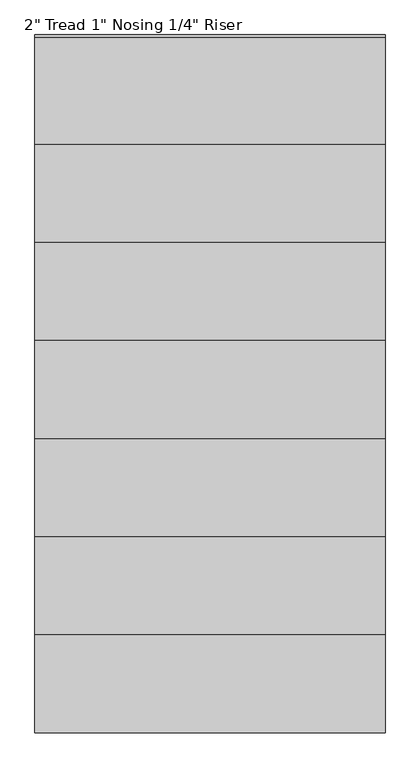
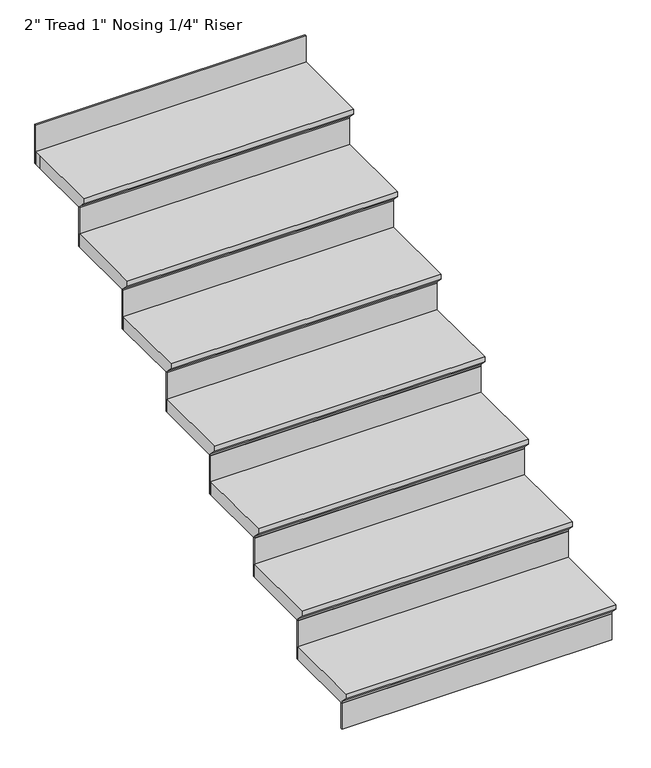
"""IFC4 building model written with IfcOpenShell, lengths in millimetres: stair flight geometry."""

from ifc_helpers import new_model, si_unit, origin, place, context, project, spatial, faceted_brep, source, transform, mapped, element, save


def stair_flight_7d9c97bb(model_context):
    return source(origin(), model_context, "Body", "Brep", [
        faceted_brep([(-6818.6502526, 9239.7128362, 3638.55), (-6818.6502526, 9239.7128362, 3657.6), (-7815.6002526, 9239.7128362, 3657.6), (-7815.6002526, 9239.7128362, 3638.55), (-6818.6502526, 9265.1128362, 3613.15), (-7815.6002526, 9265.1128362, 3613.15), (-6818.6502526, 9544.5128362, 3657.6), (-7815.6002526, 9544.5128362, 3657.6), (-7815.6002526, 9265.1128362, 3606.8), (-7815.6002526, 9544.5128362, 3606.8), (-6818.6502526, 9544.5128362, 3606.8), (-6818.6502526, 9265.1128362, 3606.8)], [[[0, 1, 2, 3]], [[4, 0, 3, 5]], [[2, 1, 6, 7]], [[8, 9, 10, 11]], [[2, 7, 9, 8, 5, 3]], [[8, 11, 4, 5]], [[6, 1, 0, 4, 11, 10]], [[7, 6, 10, 9]]]),
        faceted_brep([(-6818.6502526, 9265.1128362, 3606.8), (-6818.6502526, 9265.1128362, 3505.2), (-6818.6502526, 9271.4628362, 3505.2), (-6818.6502526, 9271.4628362, 3606.8), (-7815.6002526, 9265.1128362, 3606.8), (-7815.6002526, 9271.4628362, 3606.8), (-7815.6002526, 9271.4628362, 3505.2), (-7815.6002526, 9265.1128362, 3505.2)], [[[0, 1, 2, 3]], [[4, 5, 6, 7]], [[1, 0, 4, 7]], [[2, 1, 7, 6]], [[3, 2, 6, 5]], [[0, 3, 5, 4]]]),
        faceted_brep([(-6818.6502526, 9544.5128362, 3759.2), (-6818.6502526, 9544.5128362, 3606.8), (-6818.6502526, 9550.8628362, 3606.8), (-6818.6502526, 9550.8628362, 3759.2), (-7815.6002526, 9544.5128362, 3759.2), (-7815.6002526, 9550.8628362, 3759.2), (-7815.6002526, 9550.8628362, 3606.8), (-7815.6002526, 9544.5128362, 3606.8)], [[[0, 1, 2, 3]], [[4, 5, 6, 7]], [[1, 0, 4, 7]], [[2, 1, 7, 6]], [[3, 2, 6, 5]], [[0, 3, 5, 4]]]),
        faceted_brep([(-7815.6002526, 9519.1128362, 3810.0), (-6818.6502526, 9519.1128362, 3810.0), (-6818.6502526, 9823.9128362, 3810.0), (-7815.6002526, 9823.9128362, 3810.0), (-7815.6002526, 9544.5128362, 3759.2), (-7815.6002526, 9823.9128362, 3759.2), (-6818.6502526, 9823.9128362, 3759.2), (-6818.6502526, 9544.5128362, 3759.2), (-7815.6002526, 9544.5128362, 3765.55), (-7815.6002526, 9519.1128362, 3790.95), (-6818.6502526, 9544.5128362, 3765.55), (-6818.6502526, 9519.1128362, 3790.95)], [[[0, 1, 2, 3]], [[4, 5, 6, 7]], [[0, 3, 5, 4, 8, 9]], [[4, 7, 10, 8]], [[2, 1, 11, 10, 7, 6]], [[3, 2, 6, 5]], [[11, 1, 0, 9]], [[10, 11, 9, 8]]]),
        faceted_brep([(-6818.6502526, 9823.9128362, 3911.6), (-6818.6502526, 9823.9128362, 3759.2), (-6818.6502526, 9830.2628362, 3759.2), (-6818.6502526, 9830.2628362, 3911.6), (-7815.6002526, 9823.9128362, 3911.6), (-7815.6002526, 9830.2628362, 3911.6), (-7815.6002526, 9830.2628362, 3759.2), (-7815.6002526, 9823.9128362, 3759.2)], [[[0, 1, 2, 3]], [[4, 5, 6, 7]], [[1, 0, 4, 7]], [[2, 1, 7, 6]], [[3, 2, 6, 5]], [[0, 3, 5, 4]]]),
        faceted_brep([(-7815.6002526, 9798.5128362, 3962.4), (-6818.6502526, 9798.5128362, 3962.4), (-6818.6502526, 10103.3128362, 3962.4), (-7815.6002526, 10103.3128362, 3962.4), (-7815.6002526, 9823.9128362, 3911.6), (-7815.6002526, 10103.3128362, 3911.6), (-6818.6502526, 10103.3128362, 3911.6), (-6818.6502526, 9823.9128362, 3911.6), (-7815.6002526, 9823.9128362, 3917.95), (-7815.6002526, 9798.5128362, 3943.35), (-6818.6502526, 9823.9128362, 3917.95), (-6818.6502526, 9798.5128362, 3943.35)], [[[0, 1, 2, 3]], [[4, 5, 6, 7]], [[0, 3, 5, 4, 8, 9]], [[4, 7, 10, 8]], [[2, 1, 11, 10, 7, 6]], [[3, 2, 6, 5]], [[11, 1, 0, 9]], [[10, 11, 9, 8]]]),
        faceted_brep([(-6818.6502526, 10103.3128362, 4064.0), (-6818.6502526, 10103.3128362, 3911.6), (-6818.6502526, 10109.6628362, 3911.6), (-6818.6502526, 10109.6628362, 4064.0), (-7815.6002526, 10103.3128362, 4064.0), (-7815.6002526, 10109.6628362, 4064.0), (-7815.6002526, 10109.6628362, 3911.6), (-7815.6002526, 10103.3128362, 3911.6)], [[[0, 1, 2, 3]], [[4, 5, 6, 7]], [[1, 0, 4, 7]], [[2, 1, 7, 6]], [[3, 2, 6, 5]], [[0, 3, 5, 4]]]),
        faceted_brep([(-7815.6002526, 10077.9128362, 4114.8), (-6818.6502526, 10077.9128362, 4114.8), (-6818.6502526, 10382.7128362, 4114.8), (-7815.6002526, 10382.7128362, 4114.8), (-7815.6002526, 10103.3128362, 4064.0), (-7815.6002526, 10382.7128362, 4064.0), (-6818.6502526, 10382.7128362, 4064.0), (-6818.6502526, 10103.3128362, 4064.0), (-7815.6002526, 10103.3128362, 4070.35), (-7815.6002526, 10077.9128362, 4095.75), (-6818.6502526, 10103.3128362, 4070.35), (-6818.6502526, 10077.9128362, 4095.75)], [[[0, 1, 2, 3]], [[4, 5, 6, 7]], [[0, 3, 5, 4, 8, 9]], [[4, 7, 10, 8]], [[2, 1, 11, 10, 7, 6]], [[3, 2, 6, 5]], [[11, 1, 0, 9]], [[10, 11, 9, 8]]]),
        faceted_brep([(-6818.6502526, 10382.7128362, 4216.4), (-6818.6502526, 10382.7128362, 4064.0), (-6818.6502526, 10389.0628362, 4064.0), (-6818.6502526, 10389.0628362, 4216.4), (-7815.6002526, 10382.7128362, 4216.4), (-7815.6002526, 10389.0628362, 4216.4), (-7815.6002526, 10389.0628362, 4064.0), (-7815.6002526, 10382.7128362, 4064.0)], [[[0, 1, 2, 3]], [[4, 5, 6, 7]], [[1, 0, 4, 7]], [[2, 1, 7, 6]], [[3, 2, 6, 5]], [[0, 3, 5, 4]]]),
        faceted_brep([(-7815.6002526, 10357.3128362, 4267.2), (-6818.6502526, 10357.3128362, 4267.2), (-6818.6502526, 10662.1128362, 4267.2), (-7815.6002526, 10662.1128362, 4267.2), (-7815.6002526, 10382.7128362, 4216.4), (-7815.6002526, 10662.1128362, 4216.4), (-6818.6502526, 10662.1128362, 4216.4), (-6818.6502526, 10382.7128362, 4216.4), (-7815.6002526, 10382.7128362, 4222.75), (-7815.6002526, 10357.3128362, 4248.15), (-6818.6502526, 10382.7128362, 4222.75), (-6818.6502526, 10357.3128362, 4248.15)], [[[0, 1, 2, 3]], [[4, 5, 6, 7]], [[0, 3, 5, 4, 8, 9]], [[4, 7, 10, 8]], [[2, 1, 11, 10, 7, 6]], [[3, 2, 6, 5]], [[11, 1, 0, 9]], [[10, 11, 9, 8]]]),
        faceted_brep([(-6818.6502526, 10662.1128362, 4368.8), (-6818.6502526, 10662.1128362, 4216.4), (-6818.6502526, 10668.4628362, 4216.4), (-6818.6502526, 10668.4628362, 4368.8), (-7815.6002526, 10662.1128362, 4368.8), (-7815.6002526, 10668.4628362, 4368.8), (-7815.6002526, 10668.4628362, 4216.4), (-7815.6002526, 10662.1128362, 4216.4)], [[[0, 1, 2, 3]], [[4, 5, 6, 7]], [[1, 0, 4, 7]], [[2, 1, 7, 6]], [[3, 2, 6, 5]], [[0, 3, 5, 4]]]),
        faceted_brep([(-7815.6002526, 10636.7128362, 4419.6), (-6818.6502526, 10636.7128362, 4419.6), (-6818.6502526, 10941.5128362, 4419.6), (-7815.6002526, 10941.5128362, 4419.6), (-7815.6002526, 10662.1128362, 4368.8), (-7815.6002526, 10941.5128362, 4368.8), (-6818.6502526, 10941.5128362, 4368.8), (-6818.6502526, 10662.1128362, 4368.8), (-7815.6002526, 10662.1128362, 4375.15), (-7815.6002526, 10636.7128362, 4400.55), (-6818.6502526, 10662.1128362, 4375.15), (-6818.6502526, 10636.7128362, 4400.55)], [[[0, 1, 2, 3]], [[4, 5, 6, 7]], [[0, 3, 5, 4, 8, 9]], [[4, 7, 10, 8]], [[2, 1, 11, 10, 7, 6]], [[3, 2, 6, 5]], [[11, 1, 0, 9]], [[10, 11, 9, 8]]]),
        faceted_brep([(-6818.6502526, 11220.9128362, 4673.6), (-6818.6502526, 11220.9128362, 4521.2), (-6818.6502526, 11227.2628362, 4521.2), (-6818.6502526, 11227.2628362, 4673.6), (-7815.6002526, 11220.9128362, 4673.6), (-7815.6002526, 11227.2628362, 4673.6), (-7815.6002526, 11227.2628362, 4521.2), (-7815.6002526, 11220.9128362, 4521.2)], [[[0, 1, 2, 3]], [[4, 5, 6, 7]], [[1, 0, 4, 7]], [[2, 1, 7, 6]], [[3, 2, 6, 5]], [[0, 3, 5, 4]]]),
        faceted_brep([(-6818.6502526, 10941.5128362, 4521.2), (-6818.6502526, 10941.5128362, 4368.8), (-6818.6502526, 10947.8628362, 4368.8), (-6818.6502526, 10947.8628362, 4521.2), (-7815.6002526, 10941.5128362, 4521.2), (-7815.6002526, 10947.8628362, 4521.2), (-7815.6002526, 10947.8628362, 4368.8), (-7815.6002526, 10941.5128362, 4368.8)], [[[0, 1, 2, 3]], [[4, 5, 6, 7]], [[1, 0, 4, 7]], [[2, 1, 7, 6]], [[3, 2, 6, 5]], [[0, 3, 5, 4]]]),
        faceted_brep([(-7815.6002526, 11220.9128362, 4572.0), (-7815.6002526, 11195.5128362, 4572.0), (-7815.6002526, 10916.1128362, 4572.0), (-6818.6502526, 10916.1128362, 4572.0), (-6818.6502526, 11220.9128362, 4572.0), (-7815.6002526, 11195.5128362, 4521.2), (-7815.6002526, 11220.9128362, 4521.2), (-6818.6502526, 11220.9128362, 4521.2), (-6818.6502526, 10941.5128362, 4521.2), (-7815.6002526, 10941.5128362, 4521.2), (-7815.6002526, 10941.5128362, 4527.55), (-7815.6002526, 10916.1128362, 4552.95), (-6818.6502526, 10941.5128362, 4527.55), (-6818.6502526, 10916.1128362, 4552.95)], [[[0, 1, 2, 3, 4]], [[5, 6, 7, 8, 9]], [[1, 0, 6, 5]], [[2, 1, 5, 9, 10, 11]], [[9, 8, 12, 10]], [[4, 3, 13, 12, 8, 7]], [[0, 4, 7, 6]], [[13, 3, 2, 11]], [[12, 13, 11, 10]]]),
    ])


if __name__ == "__main__":
    model = new_model("IFC4")
    model_context = context("Model", 3, world=origin())
    ifc_project = project(units=[si_unit("LENGTHUNIT", "METRE", prefix="MILLI")], contexts=[model_context])
    site = spatial("IfcSite", under=ifc_project)
    building = spatial("IfcBuilding", under=site)
    placement = place(None, origin())
    stair_flight_shape = stair_flight_7d9c97bb(model_context)
    element("IfcStairFlight", 1, ObjectType="2\" Tread 1\" Nosing 1/4\" Riser", at=placement, inside=building, context=model_context, shape_type="MappedRepresentation", body=[
        mapped(stair_flight_shape, transform((0.0, 0.0, 0.0), x_axis=(1.0, 0.0, 0.0), y_axis=(0.0, 1.0, 0.0), z_axis=(0.0, 0.0, 1.0))),
    ])
    save(model, "model.ifc")
